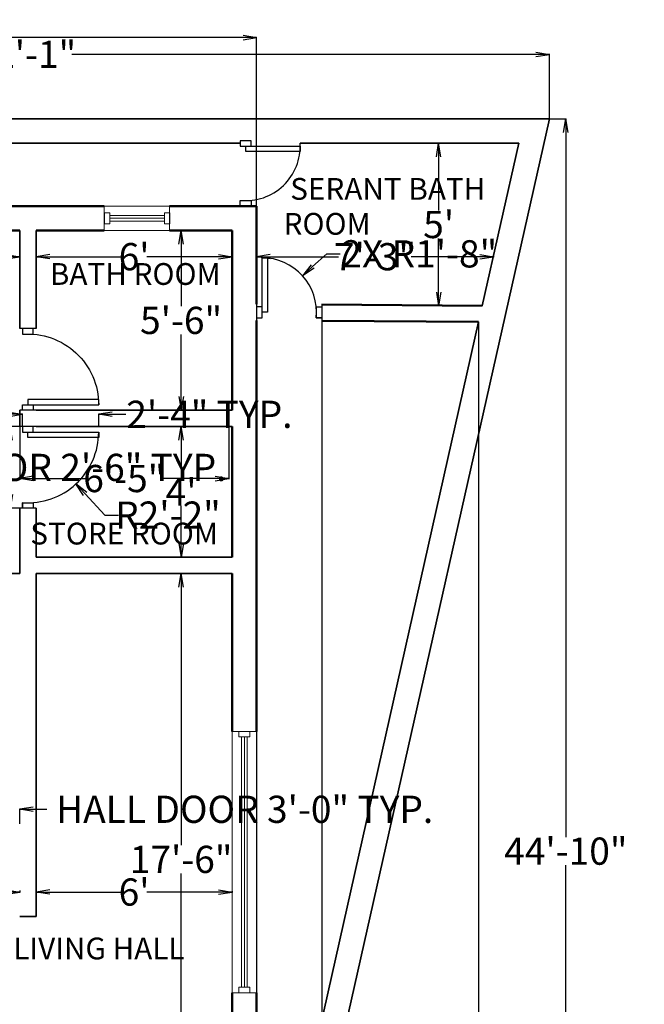
# Model space of a CAD drawing. Units: inches. Extents: x -6539 to -6057, y 19106 to 19733.
# Tile 3 of 3: x -6286 to -6057, y 19363 to 19725. Entities that reach past the tile are written whole.
import ezdxf

# ---------------------------------------------------------------- set-up
doc = ezdxf.new("R2010")
doc.units = ezdxf.units.IN
doc.header["$MEASUREMENT"] = 0
for name, color, linetype, lineweight in [('A-ANNO-DIMS', 121, 'Continuous', 18), ('A-AREA-IDEN', 250, 'Continuous', 25), ('A-WALL-EXTR', 222, 'Continuous', 50), ('C-PROP-WALL', 140, 'Continuous', 35), ('DOORS', 3, 'Continuous', 25), ('interior WALLS', 222, 'Continuous', 35), ('WINDOWS', 20, 'Continuous', 18)]:
    doc.layers.add(name, color=color, linetype=linetype, lineweight=lineweight)
doc.styles.get("Standard").update_dxf_attribs({"font": 'arial.ttf'})
doc.dimstyles.get("Standard").update_dxf_attribs({"dimtxt": 10, "dimasz": 5, "dimexe": 0.18, "dimexo": 0.0625, "dimgap": 0.09, "dimtad": 0, "dimtih": 1, "dimtoh": 1, "dimdec": 0, "dimzin": 0, "dimdsep": 46, "dimlunit": 4, "dimtxsty": 'Standard', "dimblk": 'OPEN', "dimcen": 0.09, "dimadec": 0, "dimazin": 0, "dimtfac": 1, "dimtdec": 0, "dimtofl": 0, "dimtmove": 0, "dimatfit": 0, "dimfxl": 1, "dimtolj": 1, "dimtzin": 0, "dimarcsym": 0})

# ---------------------------------------------------------------- blocks, each defined once
blk = doc.blocks.new('_Open')
at = {"color": 0, "linetype": 'ByBlock', "lineweight": -2}
for p, q in [((-1, 0.167), (0, 0)), ((-1, -0.167), (0, 0)), ((0, 0), (-1, 0))]:
    blk.add_line(p, q, dxfattribs=at)
blk = doc.blocks.new('*D2')
at = {"layer": 'A-ANNO-DIMS', "color": 0, "lineweight": -2, "transparency": 16777216}
for p, q in [((-6476.93, 19688.68), (-6476.93, 19712.48)), ((-6471.93, 19712.3), (-6301.58, 19712.3)), ((-6096.7, 19712.3), (-6267.05, 19712.3)), ((-6091.7, 19688.68), (-6091.7, 19712.48))]:
    blk.add_line(p, q, dxfattribs=at)
at = {"layer": 'Defpoints', "color": 0, "transparency": 16777216}
for p in [(-6091.7, 19712.3), (-6476.93, 19688.62), (-6091.7, 19688.62)]:
    blk.add_point(p, dxfattribs=at)
at = {"layer": 'A-ANNO-DIMS', "color": 0, "lineweight": -2, "transparency": 16777216, "xscale": 5, "yscale": 5, "zscale": 5, "rotation": 180}
blk.add_blockref('_Open', (-6476.93, 19712.3), dxfattribs=at)
at = {"layer": 'A-ANNO-DIMS', "color": 0, "lineweight": -2, "transparency": 16777216, "xscale": 5, "yscale": 5, "zscale": 5}
blk.add_blockref('_Open', (-6091.7, 19712.3), dxfattribs=at)
at = {"layer": 'A-ANNO-DIMS', "color": 0, "transparency": 16777216, "insert": (-6284.31, 19712.3), "char_height": 10, "attachment_point": 5}
blk.add_mtext('\\A1;32\'-1"', dxfattribs=at)
blk = doc.blocks.new('*D4')
at = {"layer": 'A-ANNO-DIMS', "color": 0, "lineweight": -2, "transparency": 16777216}
for p, q in [((-6091.64, 19688.62), (-6085.49, 19688.62)), ((-6085.67, 19683.62), (-6085.67, 19424.78)), ((-6085.67, 19155.56), (-6085.67, 19414.39)), ((-6212.44, 19150.56), (-6085.49, 19150.56))]:
    blk.add_line(p, q, dxfattribs=at)
at = {"layer": 'Defpoints', "color": 0, "transparency": 16777216}
for p in [(-6091.7, 19688.62), (-6085.67, 19688.62), (-6212.5, 19150.56)]:
    blk.add_point(p, dxfattribs=at)
at = {"layer": 'A-ANNO-DIMS', "color": 0, "lineweight": -2, "transparency": 16777216, "xscale": 5, "yscale": 5, "zscale": 5}
for p, rotation in [((-6085.67, 19688.62), 90), ((-6085.67, 19150.56), 270)]:
    blk.add_blockref('_Open', p, dxfattribs=dict(at, rotation=rotation))
at = {"layer": 'A-ANNO-DIMS', "color": 0, "transparency": 16777216, "insert": (-6085.67, 19419.59), "char_height": 10, "attachment_point": 5}
blk.add_mtext('\\A1;44\'-10"', dxfattribs=at)
blk = doc.blocks.new('*D6')
at = {"layer": 'A-ANNO-DIMS', "color": 0, "lineweight": -2, "transparency": 16777216}
for p, q in [((-6432.2, 19647.5), (-6432.2, 19637.79)), ((-6286.2, 19647.5), (-6286.2, 19637.79)), ((-6427.2, 19637.97), (-6376, 19637.97)), ((-6291.2, 19637.97), (-6342.41, 19637.97))]:
    blk.add_line(p, q, dxfattribs=at)
at = {"layer": 'Defpoints', "color": 0, "transparency": 16777216}
for p in [(-6432.2, 19647.56), (-6286.2, 19647.56), (-6286.2, 19637.97)]:
    blk.add_point(p, dxfattribs=at)
at = {"layer": 'A-ANNO-DIMS', "color": 0, "lineweight": -2, "transparency": 16777216, "xscale": 5, "yscale": 5, "zscale": 5, "rotation": 180}
blk.add_blockref('_Open', (-6432.2, 19637.97), dxfattribs=at)
at = {"layer": 'A-ANNO-DIMS', "color": 0, "lineweight": -2, "transparency": 16777216, "xscale": 5, "yscale": 5, "zscale": 5}
blk.add_blockref('_Open', (-6286.2, 19637.97), dxfattribs=at)
at = {"layer": 'A-ANNO-DIMS', "color": 0, "transparency": 16777216, "insert": (-6359.2, 19637.97), "char_height": 10, "attachment_point": 5}
blk.add_mtext('\\A1;12\'-2"', dxfattribs=at)
blk = doc.blocks.new('*D7')
at = {"layer": 'A-ANNO-DIMS', "color": 0, "lineweight": -2, "transparency": 16777216}
for p, q in [((-6280.2, 19637.03), (-6280.2, 19638.15)), ((-6275.2, 19637.97), (-6248.92, 19637.97)), ((-6213.2, 19637.97), (-6239.49, 19637.97)), ((-6208.2, 19638.03), (-6208.2, 19638.15))]:
    blk.add_line(p, q, dxfattribs=at)
at = {"layer": 'Defpoints', "color": 0, "transparency": 16777216}
for p in [(-6208.2, 19637.97), (-6208.2, 19637.97), (-6280.2, 19636.97)]:
    blk.add_point(p, dxfattribs=at)
at = {"layer": 'A-ANNO-DIMS', "color": 0, "lineweight": -2, "transparency": 16777216, "xscale": 5, "yscale": 5, "zscale": 5, "rotation": 180}
blk.add_blockref('_Open', (-6280.2, 19637.97), dxfattribs=at)
at = {"layer": 'A-ANNO-DIMS', "color": 0, "lineweight": -2, "transparency": 16777216, "xscale": 5, "yscale": 5, "zscale": 5}
blk.add_blockref('_Open', (-6208.2, 19637.97), dxfattribs=at)
at = {"layer": 'A-ANNO-DIMS', "color": 0, "transparency": 16777216, "insert": (-6244.2, 19637.97), "char_height": 10, "attachment_point": 5}
blk.add_mtext("\\A1;6'", dxfattribs=at)
blk = doc.blocks.new('*D8')
at = {"layer": 'A-ANNO-DIMS', "color": 0, "lineweight": -2, "transparency": 16777216}
for p, q in [((-6199.2, 19637.65), (-6199.2, 19638.15)), ((-6194.2, 19637.97), (-6169.08, 19637.97)), ((-6117.27, 19637.97), (-6142.4, 19637.97)), ((-6112.27, 19638.02), (-6112.27, 19637.79))]:
    blk.add_line(p, q, dxfattribs=at)
at = {"layer": 'Defpoints', "color": 0, "transparency": 16777216}
for p in [(-6199.2, 19637.59), (-6112.27, 19638.08), (-6112.27, 19637.97)]:
    blk.add_point(p, dxfattribs=at)
at = {"layer": 'A-ANNO-DIMS', "color": 0, "lineweight": -2, "transparency": 16777216, "xscale": 5, "yscale": 5, "zscale": 5, "rotation": 180}
blk.add_blockref('_Open', (-6199.2, 19637.97), dxfattribs=at)
at = {"layer": 'A-ANNO-DIMS', "color": 0, "lineweight": -2, "transparency": 16777216, "xscale": 5, "yscale": 5, "zscale": 5}
blk.add_blockref('_Open', (-6112.27, 19637.97), dxfattribs=at)
at = {"layer": 'A-ANNO-DIMS', "color": 0, "transparency": 16777216, "insert": (-6155.74, 19637.97), "char_height": 10, "attachment_point": 5}
blk.add_mtext('\\A1;7\'-3"', dxfattribs=at)
blk = doc.blocks.new('*D16')
at = {"layer": 'A-ANNO-DIMS', "color": 0, "lineweight": -2, "transparency": 16777216}
for p, q in [((-6432.2, 19404.62), (-6432.2, 19404.74)), ((-6427.2, 19404.56), (-6376, 19404.56)), ((-6291.2, 19404.56), (-6342.41, 19404.56)), ((-6286.2, 19405.11), (-6286.2, 19404.38))]:
    blk.add_line(p, q, dxfattribs=at)
at = {"layer": 'Defpoints', "color": 0, "transparency": 16777216}
for p in [(-6432.2, 19404.56), (-6286.2, 19405.18), (-6286.2, 19404.56)]:
    blk.add_point(p, dxfattribs=at)
at = {"layer": 'A-ANNO-DIMS', "color": 0, "lineweight": -2, "transparency": 16777216, "xscale": 5, "yscale": 5, "zscale": 5, "rotation": 180}
blk.add_blockref('_Open', (-6432.2, 19404.56), dxfattribs=at)
at = {"layer": 'A-ANNO-DIMS', "color": 0, "lineweight": -2, "transparency": 16777216, "xscale": 5, "yscale": 5, "zscale": 5}
blk.add_blockref('_Open', (-6286.2, 19404.56), dxfattribs=at)
at = {"layer": 'A-ANNO-DIMS', "color": 0, "transparency": 16777216, "insert": (-6359.2, 19404.56), "char_height": 10, "attachment_point": 5}
blk.add_mtext('\\A1;12\'-2"', dxfattribs=at)
blk = doc.blocks.new('*D17')
at = {"layer": 'A-ANNO-DIMS', "color": 0, "lineweight": -2, "transparency": 16777216}
for p, q in [((-6280.2, 19404.62), (-6280.2, 19404.74)), ((-6275.2, 19404.56), (-6248.92, 19404.56)), ((-6213.2, 19404.56), (-6239.49, 19404.56)), ((-6208.2, 19404.91), (-6208.2, 19404.38))]:
    blk.add_line(p, q, dxfattribs=at)
at = {"layer": 'Defpoints', "color": 0, "transparency": 16777216}
for p in [(-6280.2, 19404.56), (-6208.2, 19404.97), (-6208.2, 19404.56)]:
    blk.add_point(p, dxfattribs=at)
at = {"layer": 'A-ANNO-DIMS', "color": 0, "lineweight": -2, "transparency": 16777216, "xscale": 5, "yscale": 5, "zscale": 5, "rotation": 180}
blk.add_blockref('_Open', (-6280.2, 19404.56), dxfattribs=at)
at = {"layer": 'A-ANNO-DIMS', "color": 0, "lineweight": -2, "transparency": 16777216, "xscale": 5, "yscale": 5, "zscale": 5}
blk.add_blockref('_Open', (-6208.2, 19404.56), dxfattribs=at)
at = {"layer": 'A-ANNO-DIMS', "color": 0, "transparency": 16777216, "insert": (-6244.2, 19404.56), "char_height": 10, "attachment_point": 5}
blk.add_mtext("\\A1;6'", dxfattribs=at)
blk = doc.blocks.new('*D18')
at = {"layer": 'A-ANNO-DIMS', "color": 0, "lineweight": -2, "transparency": 16777216}
for p, q in [((-6103.01, 19679.62), (-6132.54, 19679.62)), ((-6132.36, 19674.62), (-6132.36, 19654.97)), ((-6132.36, 19624.97), (-6132.36, 19644.62)), ((-6116.4, 19619.97), (-6132.54, 19619.97))]:
    blk.add_line(p, q, dxfattribs=at)
at = {"layer": 'Defpoints', "color": 0, "transparency": 16777216}
for p in [(-6132.36, 19679.62), (-6102.95, 19679.62), (-6116.34, 19619.97)]:
    blk.add_point(p, dxfattribs=at)
at = {"layer": 'A-ANNO-DIMS', "color": 0, "lineweight": -2, "transparency": 16777216, "xscale": 5, "yscale": 5, "zscale": 5}
for p, rotation in [((-6132.36, 19679.62), 90), ((-6132.36, 19619.97), 270)]:
    blk.add_blockref('_Open', p, dxfattribs=dict(at, rotation=rotation))
at = {"layer": 'A-ANNO-DIMS', "color": 0, "transparency": 16777216, "insert": (-6132.36, 19649.79), "char_height": 10, "attachment_point": 5}
blk.add_mtext("\\A1;5'", dxfattribs=at)
blk = doc.blocks.new('*D19')
at = {"layer": 'A-ANNO-DIMS', "color": 0, "lineweight": -2, "transparency": 16777216}
for p, q in [((-6208.27, 19521.56), (-6227.12, 19521.56)), ((-6226.94, 19516.56), (-6226.94, 19421.75)), ((-6226.94, 19316.56), (-6226.94, 19411.36)), ((-6208.27, 19311.56), (-6227.12, 19311.56))]:
    blk.add_line(p, q, dxfattribs=at)
at = {"layer": 'Defpoints', "color": 0, "transparency": 16777216}
for p in [(-6226.94, 19521.56), (-6208.2, 19521.56), (-6208.2, 19311.56)]:
    blk.add_point(p, dxfattribs=at)
at = {"layer": 'A-ANNO-DIMS', "color": 0, "lineweight": -2, "transparency": 16777216, "xscale": 5, "yscale": 5, "zscale": 5}
for p, rotation in [((-6226.94, 19521.56), 90), ((-6226.94, 19311.56), 270)]:
    blk.add_blockref('_Open', p, dxfattribs=dict(at, rotation=rotation))
at = {"layer": 'A-ANNO-DIMS', "color": 0, "transparency": 16777216, "insert": (-6226.94, 19416.56), "char_height": 10, "attachment_point": 5}
blk.add_mtext('\\A1;17\'-6"', dxfattribs=at)
blk = doc.blocks.new('*D20')
at = {"layer": 'A-ANNO-DIMS', "color": 0, "lineweight": -2, "transparency": 16777216}
for p, q in [((-6208.27, 19575.56), (-6227.12, 19575.56)), ((-6226.94, 19570.56), (-6226.94, 19556.65)), ((-6226.94, 19532.56), (-6226.94, 19546.47)), ((-6208.27, 19527.56), (-6227.12, 19527.56))]:
    blk.add_line(p, q, dxfattribs=at)
at = {"layer": 'Defpoints', "color": 0, "transparency": 16777216}
for p in [(-6226.94, 19575.56), (-6208.2, 19575.56), (-6208.2, 19527.56)]:
    blk.add_point(p, dxfattribs=at)
at = {"layer": 'A-ANNO-DIMS', "color": 0, "lineweight": -2, "transparency": 16777216, "xscale": 5, "yscale": 5, "zscale": 5}
for p, rotation in [((-6226.94, 19575.56), 90), ((-6226.94, 19527.56), 270)]:
    blk.add_blockref('_Open', p, dxfattribs=dict(at, rotation=rotation))
at = {"layer": 'A-ANNO-DIMS', "color": 0, "transparency": 16777216, "insert": (-6226.94, 19551.56), "char_height": 10, "attachment_point": 5}
blk.add_mtext("\\A1;4'", dxfattribs=at)
blk = doc.blocks.new('*D21')
at = {"layer": 'A-ANNO-DIMS', "color": 0, "lineweight": -2, "transparency": 16777216}
for p, q in [((-6208.27, 19647.56), (-6227.12, 19647.56)), ((-6226.94, 19642.56), (-6226.94, 19619.75)), ((-6226.94, 19586.56), (-6226.94, 19609.36)), ((-6208.27, 19581.56), (-6227.12, 19581.56))]:
    blk.add_line(p, q, dxfattribs=at)
at = {"layer": 'Defpoints', "color": 0, "transparency": 16777216}
for p in [(-6226.94, 19647.56), (-6208.2, 19647.56), (-6208.2, 19581.56)]:
    blk.add_point(p, dxfattribs=at)
at = {"layer": 'A-ANNO-DIMS', "color": 0, "lineweight": -2, "transparency": 16777216, "xscale": 5, "yscale": 5, "zscale": 5}
for p, rotation in [((-6226.94, 19647.56), 90), ((-6226.94, 19581.56), 270)]:
    blk.add_blockref('_Open', p, dxfattribs=dict(at, rotation=rotation))
at = {"layer": 'A-ANNO-DIMS', "color": 0, "transparency": 16777216, "insert": (-6226.94, 19614.56), "char_height": 10, "attachment_point": 5}
blk.add_mtext('\\A1;5\'-6"', dxfattribs=at)
blk = doc.blocks.new('*D22')
at = {"layer": 'A-ANNO-DIMS', "color": 0, "lineweight": -2, "transparency": 16777216}
for p, q in [((-6286.2, 19575.5), (-6286.2, 19556.29)), ((-6209.4, 19575.5), (-6209.4, 19556.29)), ((-6281.2, 19556.47), (-6261.21, 19556.47)), ((-6214.4, 19556.47), (-6234.39, 19556.47))]:
    blk.add_line(p, q, dxfattribs=at)
at = {"layer": 'Defpoints', "color": 0, "transparency": 16777216}
for p in [(-6286.2, 19575.56), (-6209.4, 19575.56), (-6286.2, 19556.47)]:
    blk.add_point(p, dxfattribs=at)
at = {"layer": 'A-ANNO-DIMS', "color": 0, "lineweight": -2, "transparency": 16777216, "xscale": 5, "yscale": 5, "zscale": 5, "rotation": 180}
blk.add_blockref('_Open', (-6286.2, 19556.47), dxfattribs=at)
at = {"layer": 'A-ANNO-DIMS', "color": 0, "lineweight": -2, "transparency": 16777216, "xscale": 5, "yscale": 5, "zscale": 5}
blk.add_blockref('_Open', (-6209.4, 19556.47), dxfattribs=at)
at = {"layer": 'A-ANNO-DIMS', "color": 0, "transparency": 16777216, "insert": (-6247.8, 19556.47), "char_height": 10, "attachment_point": 5}
blk.add_mtext('\\A1;6\'-5"', dxfattribs=at)
blk = doc.blocks.new('DOOR-SWING-30IN')
for points in [[(0, 30), (0, 28), (4, 28), (4, 30)], [(2, 28), (28, 28), (28, 26), (2, 26)], [(0, 0), (0, 2), (4, 2), (4, 0)]]:
    blk.add_lwpolyline(points, close=True)
blk.add_arc((2, 28), 26, 265.5883, 0)
blk = doc.blocks.new('*D28')
at = {"layer": 'A-ANNO-DIMS', "color": 0, "lineweight": -2, "transparency": 16777216}
for p, q in [((-6327.2, 19434.96), (-6332.2, 19434.96)), ((-6322.2, 19429.62), (-6322.2, 19435.14)), ((-6286.2, 19429.62), (-6286.2, 19435.14)), ((-6281.2, 19434.96), (-6276.2, 19434.96))]:
    blk.add_line(p, q, dxfattribs=at)
at = {"layer": 'Defpoints', "color": 0, "transparency": 16777216}
for p in [(-6286.2, 19434.96), (-6322.2, 19429.56), (-6286.2, 19429.56)]:
    blk.add_point(p, dxfattribs=at)
at = {"layer": 'A-ANNO-DIMS', "color": 0, "lineweight": -2, "transparency": 16777216, "xscale": 5, "yscale": 5, "zscale": 5}
blk.add_blockref('_Open', (-6322.2, 19434.96), dxfattribs=at)
at = {"layer": 'A-ANNO-DIMS', "color": 0, "lineweight": -2, "transparency": 16777216, "xscale": 5, "yscale": 5, "zscale": 5, "rotation": 180}
blk.add_blockref('_Open', (-6286.2, 19434.96), dxfattribs=at)
at = {"layer": 'A-ANNO-DIMS', "color": 0, "transparency": 16777216, "insert": (-6203.6, 19434.96), "char_height": 10, "attachment_point": 5}
blk.add_mtext('\\A1;HALL DOOR 3\'-0" TYP.', dxfattribs=at)
blk = doc.blocks.new('*D30')
at = {"layer": 'A-ANNO-DIMS', "color": 0, "lineweight": -2, "transparency": 16777216}
for p, q in [((-6285.27, 19575.56), (-6289.88, 19575.56)), ((-6289.7, 19570.56), (-6289.7, 19565.82)), ((-6289.7, 19550.56), (-6289.7, 19555.29)), ((-6285.27, 19545.56), (-6289.88, 19545.56))]:
    blk.add_line(p, q, dxfattribs=at)
at = {"layer": 'Defpoints', "color": 0, "transparency": 16777216}
for p in [(-6289.7, 19575.56), (-6285.2, 19575.56), (-6285.2, 19545.56)]:
    blk.add_point(p, dxfattribs=at)
at = {"layer": 'A-ANNO-DIMS', "color": 0, "lineweight": -2, "transparency": 16777216, "xscale": 5, "yscale": 5, "zscale": 5}
for p, rotation in [((-6289.7, 19575.56), 90), ((-6289.7, 19545.56), 270)]:
    blk.add_blockref('_Open', p, dxfattribs=dict(at, rotation=rotation))
at = {"layer": 'A-ANNO-DIMS', "color": 0, "transparency": 16777216, "insert": (-6289.7, 19560.56), "char_height": 10, "attachment_point": 5}
blk.add_mtext('\\A1;SERVICE DOOR 2\'-6" TYP.', dxfattribs=at)
blk = doc.blocks.new('*D31')
at = {"layer": 'A-ANNO-DIMS', "color": 0, "lineweight": -2, "transparency": 16777216}
for p, q in [((-6290.2, 19580.06), (-6295.2, 19580.06)), ((-6285.2, 19575.62), (-6285.2, 19580.24)), ((-6257.2, 19575.62), (-6257.2, 19580.24)), ((-6252.2, 19580.06), (-6247.2, 19580.06))]:
    blk.add_line(p, q, dxfattribs=at)
at = {"layer": 'Defpoints', "color": 0, "transparency": 16777216}
for p in [(-6257.2, 19580.06), (-6285.2, 19575.56), (-6257.2, 19575.56)]:
    blk.add_point(p, dxfattribs=at)
at = {"layer": 'A-ANNO-DIMS', "color": 0, "lineweight": -2, "transparency": 16777216, "xscale": 5, "yscale": 5, "zscale": 5}
blk.add_blockref('_Open', (-6285.2, 19580.06), dxfattribs=at)
at = {"layer": 'A-ANNO-DIMS', "color": 0, "lineweight": -2, "transparency": 16777216, "xscale": 5, "yscale": 5, "zscale": 5, "rotation": 180}
blk.add_blockref('_Open', (-6257.2, 19580.06), dxfattribs=at)
at = {"layer": 'A-ANNO-DIMS', "color": 0, "transparency": 16777216, "insert": (-6216.55, 19580.06), "char_height": 10, "attachment_point": 5}
blk.add_mtext('\\A1;2\'-4" TYP.', dxfattribs=at)
blk = doc.blocks.new('*D38')
at = {"layer": 'A-ANNO-DIMS', "color": 0, "lineweight": -2, "transparency": 16777216}
for p, q in [((-6441.2, 19656.62), (-6441.2, 19718.65)), ((-6436.2, 19718.47), (-6337.56, 19718.47)), ((-6204.2, 19718.47), (-6302.85, 19718.47)), ((-6199.2, 19656.62), (-6199.2, 19718.65))]:
    blk.add_line(p, q, dxfattribs=at)
at = {"layer": 'Defpoints', "color": 0, "transparency": 16777216}
for p in [(-6199.2, 19718.47), (-6441.2, 19656.56), (-6199.2, 19656.56)]:
    blk.add_point(p, dxfattribs=at)
at = {"layer": 'A-ANNO-DIMS', "color": 0, "lineweight": -2, "transparency": 16777216, "xscale": 5, "yscale": 5, "zscale": 5, "rotation": 180}
blk.add_blockref('_Open', (-6441.2, 19718.47), dxfattribs=at)
at = {"layer": 'A-ANNO-DIMS', "color": 0, "lineweight": -2, "transparency": 16777216, "xscale": 5, "yscale": 5, "zscale": 5}
blk.add_blockref('_Open', (-6199.2, 19718.47), dxfattribs=at)
at = {"layer": 'A-ANNO-DIMS', "color": 0, "transparency": 16777216, "insert": (-6320.2, 19718.47), "char_height": 10, "attachment_point": 5}
blk.add_mtext('\\A1;20\'-2"', dxfattribs=at)
blk = doc.blocks.new('*D40')
at = {"layer": 'A-ANNO-DIMS', "color": 0, "lineweight": -2, "transparency": 16777216}
for p, q in [((-6199.2, 19614.5), (-6199.2, 19120.53)), ((-6175.2, 19614.32), (-6175.2, 19120.53)), ((-6204.2, 19120.71), (-6209.2, 19120.71)), ((-6170.2, 19120.71), (-6165.2, 19120.71))]:
    blk.add_line(p, q, dxfattribs=at)
at = {"layer": 'Defpoints', "color": 0, "transparency": 16777216}
for p in [(-6199.2, 19614.56), (-6175.2, 19614.39), (-6175.2, 19120.71)]:
    blk.add_point(p, dxfattribs=at)
at = {"layer": 'A-ANNO-DIMS', "color": 0, "lineweight": -2, "transparency": 16777216, "xscale": 5, "yscale": 5, "zscale": 5}
blk.add_blockref('_Open', (-6199.2, 19120.71), dxfattribs=at)
at = {"layer": 'A-ANNO-DIMS', "color": 0, "lineweight": -2, "transparency": 16777216, "xscale": 5, "yscale": 5, "zscale": 5, "rotation": 180}
blk.add_blockref('_Open', (-6175.2, 19120.71), dxfattribs=at)
at = {"layer": 'A-ANNO-DIMS', "color": 0, "transparency": 16777216, "insert": (-6151.74, 19120.71), "char_height": 10, "attachment_point": 5}
blk.add_mtext('\\A1;2\'-0"', dxfattribs=at)
blk = doc.blocks.new('*D41')
at = {"layer": 'A-ANNO-DIMS', "color": 0, "lineweight": -2, "transparency": 16777216}
for p, q in [((-6175.2, 19614.32), (-6175.2, 19120.53)), ((-6117.68, 19613.92), (-6117.68, 19120.53)), ((-6180.2, 19120.71), (-6185.2, 19120.71)), ((-6112.68, 19120.71), (-6107.68, 19120.71))]:
    blk.add_line(p, q, dxfattribs=at)
at = {"layer": 'Defpoints', "color": 0, "transparency": 16777216}
for p in [(-6175.2, 19614.39), (-6117.68, 19613.98), (-6117.68, 19120.71)]:
    blk.add_point(p, dxfattribs=at)
at = {"layer": 'A-ANNO-DIMS', "color": 0, "lineweight": -2, "transparency": 16777216, "xscale": 5, "yscale": 5, "zscale": 5}
blk.add_blockref('_Open', (-6175.2, 19120.71), dxfattribs=at)
at = {"layer": 'A-ANNO-DIMS', "color": 0, "lineweight": -2, "transparency": 16777216, "xscale": 5, "yscale": 5, "zscale": 5, "rotation": 180}
blk.add_blockref('_Open', (-6117.68, 19120.71), dxfattribs=at)
at = {"layer": 'A-ANNO-DIMS', "color": 0, "transparency": 16777216, "insert": (-6082.45, 19120.71), "char_height": 10, "attachment_point": 5}
blk.add_mtext('\\A1;4\'-9 1/2"', dxfattribs=at)
blk = doc.blocks.new('*D43')
at = {"layer": 'A-ANNO-DIMS', "color": 0, "lineweight": -2, "transparency": 16777216}
for p, q in [((-6283.29, 19573.56), (-6283.11, 19573.56)), ((-6283.2, 19573.47), (-6283.2, 19573.65)), ((-6262.14, 19550.81), (-6254.94, 19543.03)), ((-6254.94, 19543.03), (-6249.94, 19543.03))]:
    blk.add_line(p, q, dxfattribs=at)
at = {"layer": 'Defpoints', "color": 0, "transparency": 16777216}
for p in [(-6283.2, 19573.56), (-6265.54, 19554.48)]:
    blk.add_point(p, dxfattribs=at)
at = {"layer": 'A-ANNO-DIMS', "color": 0, "lineweight": -2, "transparency": 16777216, "xscale": 5, "yscale": 5, "zscale": 5, "rotation": 132.7932642947086}
blk.add_blockref('_Open', (-6265.54, 19554.48), dxfattribs=at)
at = {"layer": 'A-ANNO-DIMS', "color": 0, "transparency": 16777216, "insert": (-6231.78, 19543.03), "char_height": 10, "attachment_point": 5}
blk.add_mtext('\\A1;R2\'-2"', dxfattribs=at)
blk = doc.blocks.new('*D45')
at = {"layer": 'A-ANNO-DIMS', "color": 0, "lineweight": -2, "transparency": 16777216}
for p, q in [((-6178.66, 19634.33), (-6173.47, 19639.02)), ((-6173.47, 19639.02), (-6168.47, 19639.02)), ((-6197.29, 19617.56), (-6197.11, 19617.56)), ((-6197.2, 19617.47), (-6197.2, 19617.65))]:
    blk.add_line(p, q, dxfattribs=at)
at = {"layer": 'Defpoints', "color": 0, "transparency": 16777216}
for p in [(-6182.37, 19630.97), (-6197.2, 19617.56)]:
    blk.add_point(p, dxfattribs=at)
at = {"layer": 'A-ANNO-DIMS', "color": 0, "lineweight": -2, "transparency": 16777216, "xscale": 5, "yscale": 5, "zscale": 5, "rotation": 222.1310518970718}
blk.add_blockref('_Open', (-6182.37, 19630.97), dxfattribs=at)
at = {"layer": 'A-ANNO-DIMS', "color": 0, "transparency": 16777216, "insert": (-6139.48, 19639.02), "char_height": 10, "attachment_point": 5}
blk.add_mtext('\\A1;2X R1\'-8"', dxfattribs=at)

msp = doc.modelspace()

# ---------------------------------------------------------------- linework, layer by layer
at = {"layer": 'A-WALL-EXTR'}
for p, q in [((-6312.2, 19656.56), (-6255.2, 19656.56)), ((-6231.2, 19656.56), (-6199.2, 19656.56)), ((-6199.2, 19620.56), (-6199.2, 19656.56)), ((-6312.2, 19647.56), (-6286.2, 19647.56)), ((-6280.2, 19647.56), (-6255.2, 19647.56)), ((-6231.2, 19647.56), (-6208.2, 19647.56)), ((-6208.2, 19581.56), (-6208.2, 19647.56)), ((-6175.2, 19620.39), (-6116.34, 19619.97)), ((-6199.25, 19614.56), (-6199.2, 19614.56)), ((-6199.2, 19463.56), (-6199.2, 19614.56)), ((-6175.2, 19614.39), (-6117.68, 19613.98)), ((-6208.2, 19527.56), (-6208.2, 19575.56)), ((-6208.2, 19463.56), (-6208.2, 19521.56)), ((-6208.2, 19311.56), (-6208.2, 19367.56)), ((-6199.2, 19302.56), (-6199.2, 19367.56))]:
    msp.add_line(p, q, dxfattribs=at)
at = {"layer": 'C-PROP-WALL'}
for p, q in [((-6476.93, 19688.62), (-6091.7, 19688.62)), ((-6091.7, 19688.62), (-6212.5, 19150.56)), ((-6467.93, 19679.62), (-6205.2, 19679.62)), ((-6183.23, 19679.62), (-6102.95, 19679.62)), ((-6102.95, 19679.62), (-6116.34, 19619.97)), ((-6117.68, 19613.98), (-6219.7, 19159.56))]:
    msp.add_line(p, q, dxfattribs=at)
at = {"layer": 'DOORS'}
for p, q in [((-6201.2, 19680.56), (-6205.2, 19680.56)), ((-6205.2, 19680.56), (-6205.2, 19678.56)), ((-6199.2, 19656.56), (-6205.2, 19656.56)), ((-6199.2, 19620.56), (-6199.2, 19614.56)), ((-6175.2, 19620.56), (-6175.2, 19614.39)), ((-6199.2, 19615.56), (-6197.2, 19615.56)), ((-6177.3, 19615.56), (-6175.2, 19615.56)), ((-6280.2, 19611.56), (-6286.2, 19611.56)), ((-6285.2, 19581.56), (-6285.2, 19583.56)), ((-6280.2, 19581.56), (-6286.2, 19581.56)), ((-6280.2, 19575.56), (-6286.2, 19575.56)), ((-6285.2, 19575.56), (-6285.2, 19573.56)), ((-6285.2, 19547.64), (-6285.2, 19545.56)), ((-6280.2, 19545.56), (-6286.2, 19545.56))]:
    msp.add_line(p, q, dxfattribs=at)
for points in [[(-6205.2, 19680.56), (-6205.2, 19678.56), (-6201.2, 19678.56), (-6201.2, 19680.56)], [(-6203.2, 19678.56), (-6183.2, 19678.56), (-6183.2, 19676.56), (-6203.2, 19676.56)], [(-6205.2, 19656.56), (-6205.2, 19658.56), (-6201.2, 19658.56), (-6201.2, 19656.56)], [(-6197.2, 19617.56), (-6197.2, 19637.56), (-6195.2, 19637.56), (-6195.2, 19617.56)], [(-6199.2, 19615.56), (-6197.2, 19615.56), (-6197.2, 19619.56), (-6199.2, 19619.56)], [(-6175.2, 19615.56), (-6177.2, 19615.56), (-6177.2, 19619.56), (-6175.2, 19619.56)]]:
    msp.add_lwpolyline(points, close=True, dxfattribs=at)
for centre, start, end in [((-6203.2, 19678.56), 264.2608, 3.0438), ((-6197.2, 19617.56), 354.2608, 90)]:
    msp.add_arc(centre, 20, start, end, dxfattribs=at)
at = {"layer": 'interior WALLS'}
for p, q in [((-6286.2, 19611.56), (-6286.2, 19647.56)), ((-6280.2, 19611.56), (-6280.2, 19647.56)), ((-6286.2, 19575.56), (-6286.2, 19581.56)), ((-6286.2, 19575.56), (-6286.2, 19581.56)), ((-6280.2, 19581.56), (-6208.2, 19581.56)), ((-6280.2, 19575.56), (-6208.2, 19575.56)), ((-6286.2, 19521.56), (-6286.2, 19545.56)), ((-6280.2, 19527.56), (-6280.2, 19545.56)), ((-6280.2, 19527.56), (-6208.2, 19527.56)), ((-6290.2, 19521.56), (-6286.2, 19521.56)), ((-6280.2, 19395.56), (-6280.2, 19521.56)), ((-6280.2, 19521.56), (-6208.2, 19521.56)), ((-6286.2, 19395.56), (-6280.2, 19395.56))]:
    msp.add_line(p, q, dxfattribs=at)
at = {"layer": 'WINDOWS'}
for p, q in [((-6255.2, 19647.56), (-6255.2, 19656.56)), ((-6255.2, 19656.56), (-6231.06, 19656.56)), ((-6231.2, 19647.56), (-6231.2, 19656.56)), ((-6253.06, 19653.06), (-6233.06, 19653.06)), ((-6253.06, 19652.06), (-6233.06, 19652.06)), ((-6253.06, 19651.06), (-6233.06, 19651.06)), ((-6255.2, 19647.56), (-6231.06, 19647.56)), ((-6208.2, 19463.56), (-6199.2, 19463.56)), ((-6208.2, 19463.56), (-6208.2, 19367.56)), ((-6204.7, 19461.56), (-6204.7, 19369.56)), ((-6203.7, 19461.56), (-6203.7, 19369.56)), ((-6202.7, 19461.56), (-6202.7, 19369.56)), ((-6199.2, 19463.56), (-6199.2, 19367.56)), ((-6208.2, 19367.56), (-6199.2, 19367.56))]:
    msp.add_line(p, q, dxfattribs=at)
for points in [[(-6253.06, 19650.06), (-6253.06, 19654.06), (-6255.06, 19654.06), (-6255.06, 19650.06)], [(-6233.06, 19650.06), (-6233.06, 19654.06), (-6231.06, 19654.06), (-6231.06, 19650.06)], [(-6205.7, 19463.56), (-6205.7, 19461.56), (-6201.7, 19461.56), (-6201.7, 19463.56)], [(-6205.7, 19367.56), (-6205.7, 19369.56), (-6201.7, 19369.56), (-6201.7, 19367.56)]]:
    msp.add_lwpolyline(points, close=True, dxfattribs=at)

# ---------------------------------------------------------------- block references
at = {"layer": 'DOORS', "extrusion": (0, 0, -1), "zscale": -1, "rotation": 180}
msp.add_blockref('DOOR-SWING-30IN', (6285.2, 19611.56), dxfattribs=at)
at = {"layer": 'DOORS'}
msp.add_blockref('DOOR-SWING-30IN', (-6285.2, 19545.56), dxfattribs=at)

# ---------------------------------------------------------------- texts
at = {"layer": 'A-AREA-IDEN'}
for s, p in [(' SERANT BATH', (-6189.31, 19658.88)), ('ROOM', (-6189.31, 19646.03)), ('BATH ROOM ', (-6275.13, 19627.61)), ('STORE ROOM', (-6282.32, 19532.24)), ('LIVING HALL ', (-6288.56, 19379.83))]:
    msp.add_text(s, height=8, dxfattribs=at).set_placement(p)

# ---------------------------------------------------------------- dimensions: what is measured, and where the dimension line sits
at = {"layer": 'A-ANNO-DIMS'}
for base, p1, p2, override, picture, middle in [((-6199.2, 19718.47), (-6441.2, 19656.56), (-6199.2, 19656.56), {"dimdec": 1, "dimlfac": 1, "dimrnd": 0, "dimzin": 1, "dimdsep": 46, "dimlunit": 4, "dimfrac": 2}, '*D38', (-6320.2, 19718.47)), ((-6091.7, 19712.3), (-6476.93, 19688.62), (-6091.7, 19688.62), {"dimclrd": 0, "dimclre": 0, "dimclrt": 0}, '*D2', (-6284.31, 19712.3)), ((-6286.2, 19637.97), (-6432.2, 19647.56), (-6286.2, 19647.56), {"dimclrd": 0, "dimclre": 0, "dimclrt": 0}, '*D6', (-6359.2, 19637.97)), ((-6208.2, 19637.97), (-6280.2, 19636.97), (-6208.2, 19637.97), {"dimclrd": 0, "dimclre": 0, "dimclrt": 0, "dimtmove": 1}, '*D7', (-6244.2, 19637.97)), ((-6112.27, 19637.97), (-6199.2, 19637.59), (-6112.27, 19638.08), {"dimclrd": 0, "dimclre": 0, "dimclrt": 0, "dimtmove": 1}, '*D8', (-6155.74, 19637.97)), ((-6175.2, 19120.71), (-6199.2, 19614.56), (-6175.2, 19614.39), {"dimdec": 1, "dimlfac": 1, "dimrnd": 0, "dimzin": 1, "dimdsep": 46, "dimlunit": 4, "dimfrac": 2}, '*D40', (-6151.74, 19120.71)), ((-6117.68, 19120.71), (-6175.2, 19614.39), (-6117.68, 19613.98), {"dimdec": 1, "dimlfac": 1, "dimrnd": 0, "dimzin": 1, "dimdsep": 46, "dimlunit": 4, "dimfrac": 2}, '*D41', (-6082.45, 19120.71)), ((-6286.2, 19556.47), (-6209.4, 19575.56), (-6286.2, 19575.56), {"dimclrd": 0, "dimclre": 0, "dimclrt": 0}, '*D22', (-6247.8, 19556.47)), ((-6286.2, 19404.56), (-6432.2, 19404.56), (-6286.2, 19405.18), {"dimclrd": 0, "dimclre": 0, "dimclrt": 0}, '*D16', (-6359.2, 19404.56)), ((-6208.2, 19404.56), (-6280.2, 19404.56), (-6208.2, 19404.97), {"dimclrd": 0, "dimclre": 0, "dimclrt": 0, "dimtmove": 1}, '*D17', (-6244.2, 19404.56))]:
    dim = msp.add_linear_dim(base=base, p1=p1, p2=p2, dimstyle='Standard', override=override, dxfattribs=at)
    dim.commit()
    dim.dimension.update_dxf_attribs({"geometry": picture, "text_midpoint": middle})
for base, p1, p2, override, picture, middle in [((-6085.67, 19688.62), (-6212.5, 19150.56), (-6091.7, 19688.62), {"dimclrd": 0, "dimclre": 0, "dimclrt": 0}, '*D4', (-6085.67, 19419.59)), ((-6132.36, 19679.62), (-6116.34, 19619.97), (-6102.95, 19679.62), {"dimclrd": 0, "dimclre": 0, "dimclrt": 0}, '*D18', (-6132.36, 19649.79)), ((-6226.94, 19647.56), (-6208.2, 19581.56), (-6208.2, 19647.56), {"dimclrd": 0, "dimclre": 0, "dimclrt": 0, "dimtmove": 1}, '*D21', (-6226.94, 19614.56)), ((-6226.94, 19575.56), (-6208.2, 19527.56), (-6208.2, 19575.56), {"dimclrd": 0, "dimclre": 0, "dimclrt": 0, "dimtmove": 1}, '*D20', (-6226.94, 19551.56)), ((-6226.94, 19521.56), (-6208.2, 19311.56), (-6208.2, 19521.56), {"dimclrd": 0, "dimclre": 0, "dimclrt": 0}, '*D19', (-6226.94, 19416.56))]:
    dim = msp.add_linear_dim(base=base, p1=p1, p2=p2, angle=90, dimstyle='Standard', override=override, dxfattribs=at)
    dim.commit()
    dim.dimension.update_dxf_attribs({"geometry": picture, "text_midpoint": middle})
dim = msp.add_radius_dim(center=(-6197.2, 19617.56), mpoint=(-6182.37, 19630.97), text='2X <>', dimstyle='Standard', override={"dimdec": 1, "dimlfac": 1, "dimrnd": 0, "dimzin": 1, "dimdsep": 46, "dimlunit": 4, "dimfrac": 2}, dxfattribs=at)
dim.commit()
dim.dimension.update_dxf_attribs({"geometry": '*D45', "text_midpoint": (-6139.48, 19639.02), "dimtype": 164})
for base, p1, p2, text, picture, middle in [((-6257.2, 19580.06), (-6285.2, 19575.56), (-6257.2, 19575.56), '<> TYP.', '*D31', (-6216.55, 19580.06)), ((-6286.2, 19434.96), (-6322.2, 19429.56), (-6286.2, 19429.56), 'HALL DOOR <> TYP.', '*D28', (-6203.6, 19434.96))]:
    dim = msp.add_linear_dim(base=base, p1=p1, p2=p2, text=text, dimstyle='Standard', override={"dimdec": 1, "dimlfac": 1, "dimrnd": 0, "dimzin": 1, "dimdsep": 46, "dimlunit": 4, "dimfrac": 2}, dxfattribs=at)
    dim.commit()
    dim.dimension.update_dxf_attribs({"geometry": picture, "text_midpoint": middle})
dim = msp.add_linear_dim(base=(-6289.7, 19575.56), p1=(-6285.2, 19545.56), p2=(-6285.2, 19575.56), angle=90, text='SERVICE DOOR <> TYP.', dimstyle='Standard', override={"dimdec": 1, "dimlfac": 1, "dimrnd": 0, "dimzin": 1, "dimdsep": 46, "dimlunit": 4, "dimfrac": 2}, dxfattribs=at)
dim.commit()
dim.dimension.update_dxf_attribs({"geometry": '*D30', "text_midpoint": (-6289.7, 19560.56)})
dim = msp.add_radius_dim(center=(-6283.2, 19573.56), mpoint=(-6265.54, 19554.48), dimstyle='Standard', override={"dimdec": 1, "dimlfac": 1, "dimrnd": 0, "dimzin": 1, "dimdsep": 46, "dimlunit": 4, "dimfrac": 2}, dxfattribs=at)
dim.commit()
dim.dimension.update_dxf_attribs({"geometry": '*D43', "text_midpoint": (-6231.78, 19543.03), "dimtype": 164})

doc.saveas('drawing.dxf')
